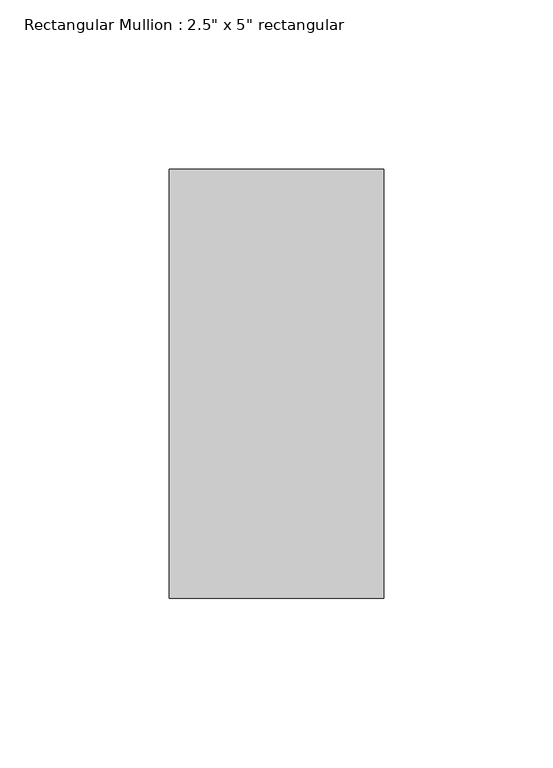
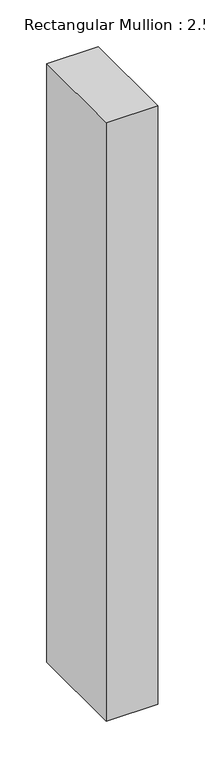
"""IFC4 building model written with IfcOpenShell, lengths in millimetres: member geometry."""

from ifc_helpers import new_model, si_unit, frame, origin, place, context, project, spatial, polyline, outline, extrude, source, transform, mapped, element, save


def member_44fc35f8(model_context):
    return source(origin(), model_context, "Body", "SweptSolid", [
        extrude(outline(polyline([(31.75, 63.5), (31.75, -63.5), (-31.75, -63.5), (-31.75, 63.5), (31.75, 63.5)])), frame((0.0, 0.0, -780.2809615), z_axis=(0.0, 0.0, 1.0), x_axis=(1.0, 0.0, 0.0)), (0.0, 0.0, 1.0), 780.2809615),
    ])


if __name__ == "__main__":
    model = new_model("IFC4")
    model_context = context("Model", 3, world=origin())
    ifc_project = project(units=[si_unit("LENGTHUNIT", "METRE", prefix="MILLI")], contexts=[model_context])
    site = spatial("IfcSite", under=ifc_project)
    building = spatial("IfcBuilding", under=site)
    placement = place(None, origin())
    member_shape = member_44fc35f8(model_context)
    element("IfcMember", 1, ObjectType="Rectangular Mullion : 2.5\" x 5\" rectangular", at=placement, inside=building, context=model_context, shape_type="MappedRepresentation", body=[
        mapped(member_shape, transform((0.0, 0.0, 0.0), x_axis=(1.0, 0.0, 0.0), y_axis=(0.0, 1.0, 0.0), z_axis=(0.0, 0.0, 1.0))),
    ])
    save(model, "model.ifc")

# Revit data of these elements
# Type "Rectangular Mullion : 2.5\" x 5\" rectangular"
#   built-in parameter 1007304 = 0.416667 (stored number, unit not read)
#   built-in parameter 1007301 = 0.104167 (stored number, unit not read)
#   built-in parameter 1007300 = 0.104167 (stored number, unit not read)
# Element 1 (IfcMember, "Rectangular Mullion : 2.5\" x 5\" rectangular")
#   Materials on its faces: "Aluminum"
# Materials
#   "Aluminum": class "Metal", colour RGB 247 247 247, transparency 0, Description = "Aluminum 6061", Cost = 0
